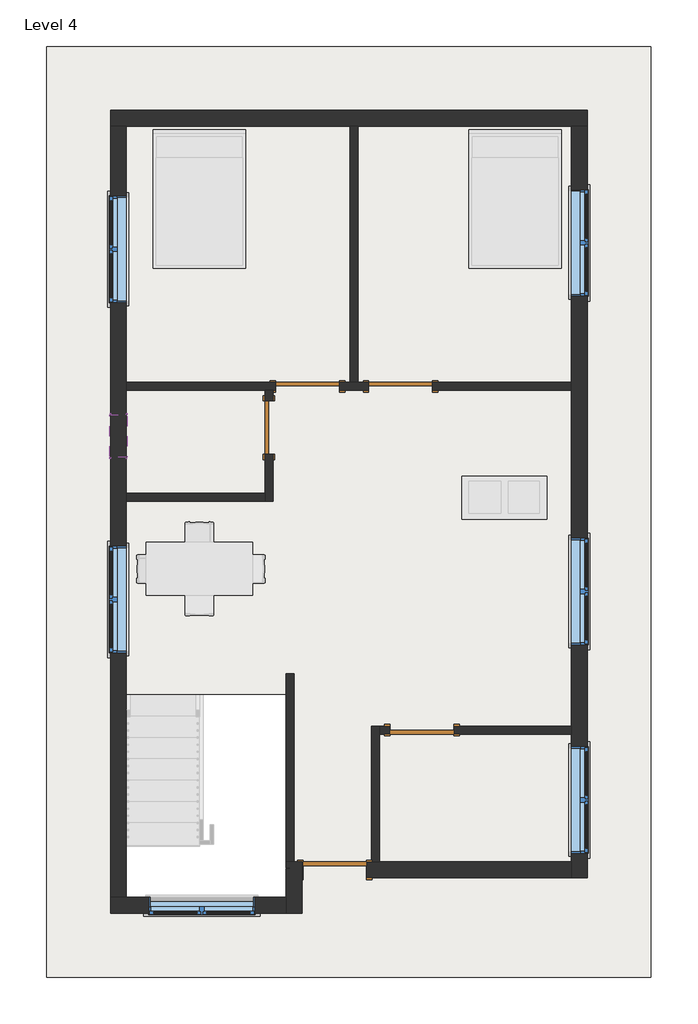
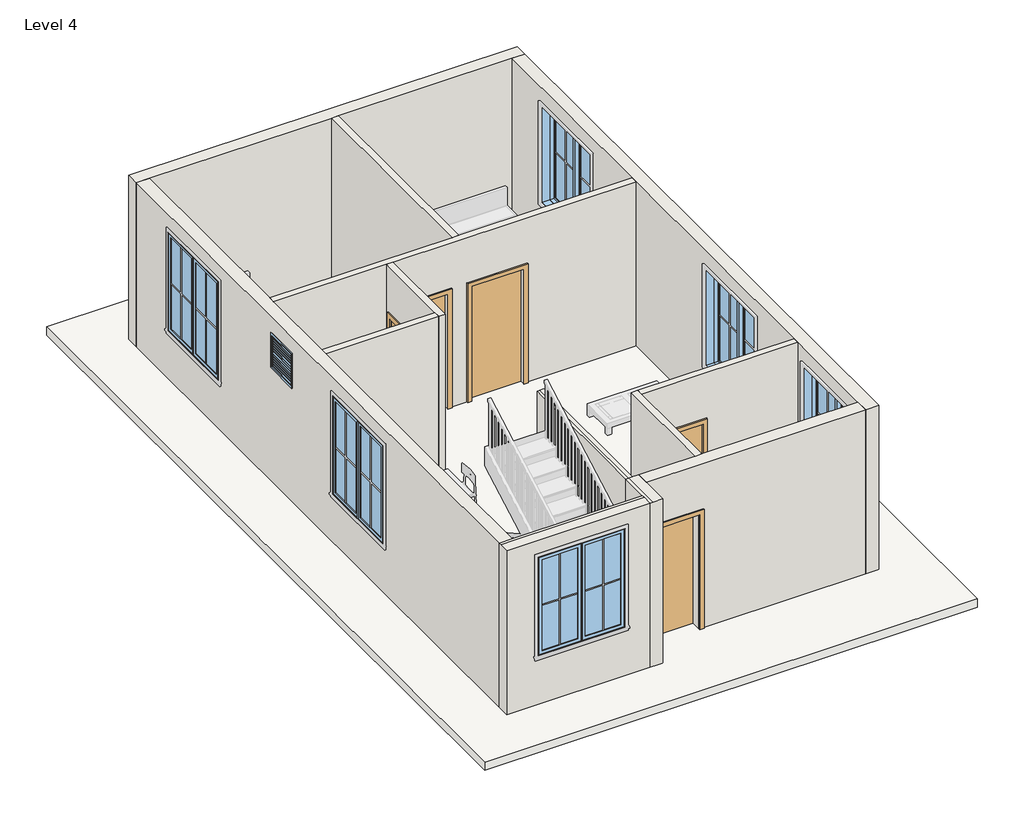
# One storey, part 1 of 3: 13 walls, 7 windows, 5 doors, 1 roof.
"""IFC4 building model written with IfcOpenShell, lengths in millimetres."""

from ifc_helpers import new_model, si_unit, frame, origin, place, context, project, spatial, polyline, outline, extrude, faceted_brep, transform, mapped, element, save
from components import door_214872d5, single_flush_door_3_e5f9f3c4, single_flush_door_3_305aa2a5, single_flush_door_3_0ca8825f, window_casement_double_win_5_f93960c7, window_f2d8fef0

model = new_model("IFC4")

# Units and contexts
model_context = context("Model", 3, world=origin())
ifc_project = project(units=[si_unit("LENGTHUNIT", "METRE", prefix="MILLI")], contexts=[model_context])

# Site, building, storey
site = spatial("IfcSite", under=ifc_project)
building = spatial("IfcBuilding", under=site)
storey = spatial("IfcBuildingStorey", under=building, Name="Level 4", Elevation=9448.8)

# Doors
placement = place(None, origin())
door_shape = door_214872d5(model_context)
element("IfcDoor", 1, ObjectType="Single-Flush : DOOR 2'6\"", at=placement, inside=storey, context=model_context, shape_type="MappedRepresentation", body=[
    mapped(door_shape, transform((-2193.930864, 251.0919982, 9448.8), x_axis=(0.0, 1.0, 0.0), y_axis=(-1.0, 0.0, 0.0), z_axis=(0.0, 0.0, 1.0))),
])
single_flush_door_3_shape = single_flush_door_3_e5f9f3c4(model_context)
element("IfcDoor", 2, ObjectType="Single-Flush : DOOR 3'", at=placement, inside=storey, context=model_context, shape_type="MappedRepresentation", body=[
    mapped(single_flush_door_3_shape, transform((-1641.3962678, 841.6419982, 9448.8), x_axis=(1.0, 0.0, 0.0), y_axis=(0.0, 1.0, 0.0), z_axis=(0.0, 0.0, 1.0))),
])
element("IfcDoor", 3, ObjectType="Single-Flush : DOOR 3'", at=placement, inside=storey, context=model_context, shape_type="MappedRepresentation", body=[
    mapped(single_flush_door_3_shape, transform((-3.180864, -4073.2580018, 9448.8), x_axis=(-1.0, 0.0, 0.0), y_axis=(0.0, -1.0, 0.0), z_axis=(0.0, 0.0, 1.0))),
])
single_flush_door_3_2_shape = single_flush_door_3_305aa2a5(model_context)
element("IfcDoor", 4, ObjectType="Single-Flush : DOOR 3'", at=placement, inside=storey, context=model_context, shape_type="MappedRepresentation", body=[
    mapped(single_flush_door_3_2_shape, transform((-307.980864, 841.6419982, 9448.8), x_axis=(-1.0, 0.0, 0.0), y_axis=(0.0, -1.0, 0.0), z_axis=(0.0, 0.0, 1.0))),
])
single_flush_door_3_3_shape = single_flush_door_3_0ca8825f(model_context)
element("IfcDoor", 5, ObjectType="Single-Flush : DOOR 3'", at=placement, inside=storey, context=model_context, shape_type="MappedRepresentation", body=[
    mapped(single_flush_door_3_3_shape, transform((-1250.955864, -6073.5080018, 9448.8), x_axis=(1.0, 0.0, 0.0), y_axis=(0.0, 1.0, 0.0), z_axis=(0.0, 0.0, 1.0))),
])

# Roof
element("IfcRoof", 6, ObjectType="ROOF 6\"", at=placement, inside=storey, context=model_context, shape_type="SweptSolid", body=[
    extrude(outline(polyline([(3273.419136, 5699.3919982), (3273.419136, -7610.2080018), (-5375.280864, -7610.2080018), (-5375.280864, 5699.3919982), (3273.419136, 5699.3919982)]), holes=[polyline([(-1895.480864, -3571.6080018), (-4232.280864, -3571.6080018), (-4232.280864, -6518.0080018), (-1895.480864, -6518.0080018), (-1895.480864, -3571.6080018)])]), frame((0.0, 0.0, 9296.4), z_axis=(0.0, 0.0, 1.0), x_axis=(1.0, 0.0, 0.0)), (0.0, 0.0, 1.0), 152.4),
])

# Walls
element("IfcWall", 7, ObjectType="WALL 4.5\"", at=placement, inside=storey, context=model_context, shape_type="SweptSolid", body=[
    extrude(outline(polyline([(-1031.880864, 898.7919982), (-1031.880864, 4556.3919982), (-917.580864, 4556.3919982), (-917.580864, 898.7919982), (-1031.880864, 898.7919982)])), frame((0.0, 0.0, 9448.8), z_axis=(0.0, 0.0, 1.0), x_axis=(1.0, 0.0, 0.0)), (0.0, 0.0, 1.0), 3048.0),
])
element("IfcWall", 8, ObjectType="WALL 4.5\"", at=placement, inside=storey, context=model_context, shape_type="Brep", body=[
    faceted_brep([(-765.180864, 898.7919982, 11582.4), (-765.180864, 898.7919982, 9448.8), (-917.580864, 898.7919982, 9448.8), (-1031.880864, 898.7919982, 9448.8), (-1184.1962678, 898.7919982, 9448.8), (-1184.1962678, 898.7919982, 11582.4), (-2098.5962678, 898.7919982, 11582.4), (-2098.5962678, 898.7919982, 9448.8), (-4232.280864, 898.7919982, 9448.8), (-4232.280864, 898.7919982, 12496.8), (-1031.880864, 898.7919982, 12496.8), (-917.580864, 898.7919982, 12496.8), (2130.419136, 898.7919982, 12496.8), (2130.419136, 898.7919982, 9448.8), (149.219136, 898.7919982, 9448.8), (149.219136, 898.7919982, 11582.4), (-1184.1962678, 784.4919982, 9448.8), (-765.180864, 784.4919982, 9448.8), (-765.180864, 784.4919982, 11582.4), (149.219136, 784.4919982, 11582.4), (149.219136, 784.4919982, 9448.8), (2130.419136, 784.4919982, 9448.8), (2130.419136, 784.4919982, 12496.8), (-2136.780864, 784.4919982, 12496.8), (-2251.080864, 784.4919982, 12496.8), (-4232.280864, 784.4919982, 12496.8), (-4232.280864, 784.4919982, 9448.8), (-2251.080864, 784.4919982, 9448.8), (-2136.780864, 784.4919982, 9448.8), (-2098.5962678, 784.4919982, 9448.8), (-2098.5962678, 784.4919982, 11582.4), (-1184.1962678, 784.4919982, 11582.4)], [[[0, 1, 2, 3, 4, 5, 6, 7, 8, 9, 10, 11, 12, 13, 14, 15]], [[16, 17, 18, 19, 20, 21, 22, 23, 24, 25, 26, 27, 28, 29, 30, 31]], [[29, 28, 27, 26, 8, 7]], [[14, 13, 21, 20]], [[4, 3, 2, 1, 17, 16]], [[13, 12, 22, 21]], [[9, 8, 26, 25]], [[5, 4, 16, 31]], [[6, 5, 31, 30]], [[7, 6, 30, 29]], [[18, 17, 1, 0]], [[19, 18, 0, 15]], [[20, 19, 15, 14]], [[12, 11, 10, 9, 25, 24, 23, 22]]]),
])
element("IfcWall", 9, ObjectType="WALL 4.5\"", at=placement, inside=storey, context=model_context, shape_type="Brep", body=[
    faceted_brep([(-2251.080864, 784.4919982, 9448.8), (-2251.080864, 632.0919982, 9448.8), (-2251.080864, 632.0919982, 11582.4), (-2251.080864, -129.9080018, 11582.4), (-2251.080864, -129.9080018, 9448.8), (-2251.080864, -688.7080018, 9448.8), (-2251.080864, -803.0080018, 9448.8), (-2251.080864, -803.0080018, 12496.8), (-2251.080864, -688.7080018, 12496.8), (-2251.080864, 784.4919982, 12496.8), (-2136.780864, 632.0919982, 11582.4), (-2136.780864, 632.0919982, 9448.8), (-2136.780864, 784.4919982, 9448.8), (-2136.780864, 784.4919982, 12496.8), (-2136.780864, -803.0080018, 12496.8), (-2136.780864, -803.0080018, 9448.8), (-2136.780864, -129.9080018, 9448.8), (-2136.780864, -129.9080018, 11582.4)], [[[0, 1, 2, 3, 4, 5, 6, 7, 8, 9]], [[10, 11, 12, 13, 14, 15, 16, 17]], [[16, 15, 6, 5, 4]], [[12, 11, 1, 0]], [[0, 9, 13, 12]], [[7, 6, 15, 14]], [[2, 1, 11, 10]], [[3, 2, 10, 17]], [[4, 3, 17, 16]], [[9, 8, 7, 14, 13]]]),
])
element("IfcWall", 10, ObjectType="WALL 4.5\"", at=placement, inside=storey, context=model_context, shape_type="SweptSolid", body=[
    extrude(outline(polyline([(-4232.280864, -688.7080018), (-2251.080864, -688.7080018), (-2251.080864, -803.0080018), (-4232.280864, -803.0080018), (-4232.280864, -688.7080018)])), frame((0.0, 0.0, 9448.8), z_axis=(0.0, 0.0, 1.0), x_axis=(1.0, 0.0, 0.0)), (0.0, 0.0, 1.0), 3048.0),
])
element("IfcWall", 11, ObjectType="WALL 4.5\"", at=placement, inside=storey, context=model_context, shape_type="Brep", body=[
    faceted_brep([(-1831.980864, -5959.2080018, 9448.8), (-1831.980864, -3266.8080018, 9448.8), (-1831.980864, -3266.8080018, 12496.8), (-1831.980864, -5959.2080018, 12496.8), (-1946.280864, -5959.2080018, 9448.8), (-1946.280864, -5959.2080018, 12496.8), (-1946.280864, -3266.8080018, 12496.8), (-1946.280864, -3266.8080018, 9448.8), (-1895.480864, -3266.8080018, 12496.8), (-1895.480864, -5959.2080018, 12496.8), (-1895.480864, -3571.6080018, 12496.8)], [[[0, 1, 2, 3]], [[4, 5, 6, 7]], [[1, 0, 4, 7]], [[2, 1, 7, 6, 8]], [[0, 3, 9, 5, 4]], [[3, 2, 8, 10, 9]], [[8, 6, 5, 9, 10]]]),
])
element("IfcWall", 12, ObjectType="WALL 4.5\"", at=placement, inside=storey, context=model_context, shape_type="Brep", body=[
    faceted_brep([(-612.780864, -5959.2080018, 9448.8), (-612.780864, -4130.4080018, 9448.8), (-612.780864, -4016.1080018, 9448.8), (-612.780864, -4016.1080018, 12496.8), (-612.780864, -4130.4080018, 12496.8), (-612.780864, -5959.2080018, 12496.8), (-727.080864, -5959.2080018, 9448.8), (-727.080864, -5959.2080018, 12496.8), (-727.080864, -4016.1080018, 12496.8), (-727.080864, -4016.1080018, 9448.8)], [[[0, 1, 2, 3, 4, 5]], [[6, 7, 8, 9]], [[2, 1, 0, 6, 9]], [[0, 5, 7, 6]], [[3, 2, 9, 8]], [[5, 4, 3, 8, 7]]]),
])
element("IfcWall", 13, ObjectType="WALL 4.5\"", at=placement, inside=storey, context=model_context, shape_type="SweptSolid", body=[
    extrude(outline(polyline([(9448.8, -612.780864), (9448.8, -460.380864), (11582.4, -460.380864), (11582.4, 454.019136), (9448.8, 454.019136), (9448.8, 2130.419136), (12496.8, 2130.419136), (12496.8, -612.780864), (9448.8, -612.780864)])), frame((0.0, -4130.4080018, 0.0), z_axis=(0.0, 1.0, 0.0), x_axis=(0.0, 0.0, 1.0)), (0.0, 0.0, 1.0), 114.3),
])
element("IfcWall", 14, ObjectType="WALL 9\"", at=placement, inside=storey, context=model_context, shape_type="Brep", body=[
    faceted_brep([(-4460.880864, 4556.3919982, 9448.8), (-4232.280864, 4556.3919982, 9448.8), (-1031.880864, 4556.3919982, 9448.8), (-917.580864, 4556.3919982, 9448.8), (2130.419136, 4556.3919982, 9448.8), (2359.019136, 4556.3919982, 9448.8), (2359.019136, 4556.3919982, 12496.8), (2130.419136, 4556.3919982, 12496.8), (-917.580864, 4556.3919982, 12496.8), (-1031.880864, 4556.3919982, 12496.8), (-4232.280864, 4556.3919982, 12496.8), (-4460.880864, 4556.3919982, 12496.8), (-4460.880864, 4784.9919982, 9448.8), (-4460.880864, 4784.9919982, 12496.8), (2359.019136, 4784.9919982, 12496.8), (2359.019136, 4784.9919982, 9448.8)], [[[0, 1, 2, 3, 4, 5, 6, 7, 8, 9, 10, 11]], [[12, 13, 14, 15]], [[5, 4, 3, 2, 1, 0, 12, 15]], [[6, 5, 15, 14]], [[0, 11, 13, 12]], [[11, 10, 9, 8, 7, 6, 14, 13]]]),
])
element("IfcWall", 15, ObjectType="WALL 9\"", at=placement, inside=storey, context=model_context, shape_type="Brep", body=[
    faceted_brep([(2130.419136, 4556.3919982, 9448.8), (2130.419136, 898.7919982, 9448.8), (2130.419136, 784.4919982, 9448.8), (2130.419136, -4016.1080018, 9448.8), (2130.419136, -4130.4080018, 9448.8), (2130.419136, -5959.2080018, 9448.8), (2130.419136, -6187.8080018, 9448.8), (2130.419136, -6187.8080018, 12496.8), (2130.419136, -5959.2080018, 12496.8), (2130.419136, -4130.4080018, 12496.8), (2130.419136, -4016.1080018, 12496.8), (2130.419136, 784.4919982, 12496.8), (2130.419136, 898.7919982, 12496.8), (2130.419136, 4556.3919982, 12496.8), (2130.419136, -5835.3830018, 12192.0), (2130.419136, -5835.3830018, 10363.2), (2130.419136, -4311.3830018, 10363.2), (2130.419136, -4311.3830018, 12192.0), (2130.419136, -2854.0580018, 12192.0), (2130.419136, -2854.0580018, 10363.2), (2130.419136, -1330.0580018, 10363.2), (2130.419136, -1330.0580018, 12192.0), (2130.419136, 2130.6919982, 12192.0), (2130.419136, 2130.6919982, 10363.2), (2130.419136, 3654.6919982, 10363.2), (2130.419136, 3654.6919982, 12192.0), (2359.019136, 4556.3919982, 9448.8), (2359.019136, 4556.3919982, 12496.8), (2359.019136, -6187.8080018, 12496.8), (2359.019136, -6187.8080018, 9448.8), (2359.019136, -5835.3830018, 12192.0), (2359.019136, -4311.3830018, 12192.0), (2359.019136, -4311.3830018, 10363.2), (2359.019136, -5835.3830018, 10363.2), (2359.019136, -2854.0580018, 12192.0), (2359.019136, -1330.0580018, 12192.0), (2359.019136, -1330.0580018, 10363.2), (2359.019136, -2854.0580018, 10363.2), (2359.019136, 2130.6919982, 12192.0), (2359.019136, 3654.6919982, 12192.0), (2359.019136, 3654.6919982, 10363.2), (2359.019136, 2130.6919982, 10363.2)], [[[0, 1, 2, 3, 4, 5, 6, 7, 8, 9, 10, 11, 12, 13], [14, 15, 16, 17], [18, 19, 20, 21], [22, 23, 24, 25]], [[26, 27, 28, 29], [30, 31, 32, 33], [34, 35, 36, 37], [38, 39, 40, 41]], [[6, 5, 4, 3, 2, 1, 0, 26, 29]], [[0, 13, 27, 26]], [[7, 6, 29, 28]], [[15, 14, 30, 33]], [[16, 15, 33, 32]], [[17, 16, 32, 31]], [[14, 17, 31, 30]], [[19, 18, 34, 37]], [[20, 19, 37, 36]], [[21, 20, 36, 35]], [[18, 21, 35, 34]], [[23, 22, 38, 41]], [[24, 23, 41, 40]], [[25, 24, 40, 39]], [[22, 25, 39, 38]], [[13, 12, 11, 10, 9, 8, 7, 28, 27]]]),
])
element("IfcWall", 16, ObjectType="WALL 9\"", at=placement, inside=storey, context=model_context, shape_type="Brep", body=[
    faceted_brep([(2130.419136, -5959.2080018, 9448.8), (-612.780864, -5959.2080018, 9448.8), (-727.080864, -5959.2080018, 9448.8), (-793.755864, -5959.2080018, 9448.8), (-793.755864, -5959.2080018, 11582.4), (-1708.155864, -5959.2080018, 11582.4), (-1708.155864, -5959.2080018, 9448.8), (-1717.680864, -5959.2080018, 9448.8), (-1717.680864, -5959.2080018, 12496.8), (-727.080864, -5959.2080018, 12496.8), (-612.780864, -5959.2080018, 12496.8), (2130.419136, -5959.2080018, 12496.8), (-793.755864, -6187.8080018, 11582.4), (-793.755864, -6187.8080018, 9448.8), (2130.419136, -6187.8080018, 9448.8), (2130.419136, -6187.8080018, 12496.8), (-1717.680864, -6187.8080018, 12496.8), (-1717.680864, -6187.8080018, 9448.8), (-1708.155864, -6187.8080018, 9448.8), (-1708.155864, -6187.8080018, 11582.4)], [[[0, 1, 2, 3, 4, 5, 6, 7, 8, 9, 10, 11]], [[12, 13, 14, 15, 16, 17, 18, 19]], [[18, 17, 7, 6]], [[14, 13, 3, 2, 1, 0]], [[0, 11, 15, 14]], [[8, 7, 17, 16]], [[4, 3, 13, 12]], [[5, 4, 12, 19]], [[6, 5, 19, 18]], [[11, 10, 9, 8, 16, 15]]]),
])
element("IfcWall", 17, ObjectType="WALL 9\"", at=placement, inside=storey, context=model_context, shape_type="Brep", body=[
    faceted_brep([(-1946.280864, -5959.2080018, 9448.8), (-1946.280864, -6467.2080018, 9448.8), (-1946.280864, -6695.8080018, 9448.8), (-1946.280864, -6695.8080018, 12496.8), (-1946.280864, -6467.2080018, 12496.8), (-1946.280864, -5959.2080018, 12496.8), (-1717.680864, -5959.2080018, 9448.8), (-1717.680864, -5959.2080018, 12496.8), (-1717.680864, -6187.8080018, 12496.8), (-1717.680864, -6695.8080018, 12496.8), (-1717.680864, -6695.8080018, 9448.8), (-1717.680864, -6187.8080018, 9448.8), (-1831.980864, -5959.2080018, 9448.8), (-1895.480864, -5959.2080018, 12496.8), (-1831.980864, -5959.2080018, 12496.8), (-1895.480864, -6695.8080018, 12496.8), (-1895.480864, -6518.0080018, 12496.8)], [[[0, 1, 2, 3, 4, 5]], [[6, 7, 8, 9, 10, 11]], [[2, 1, 0, 12, 6, 11, 10]], [[0, 5, 13, 14, 7, 6, 12]], [[3, 2, 10, 9, 15]], [[5, 4, 3, 15, 16, 13]], [[15, 9, 8, 7, 14, 13, 16]]]),
])
element("IfcWall", 18, ObjectType="WALL 9\"", at=placement, inside=storey, context=model_context, shape_type="Brep", body=[
    faceted_brep([(-1946.280864, -6467.2080018, 9448.8), (-4232.280864, -6467.2080018, 9448.8), (-4460.880864, -6467.2080018, 9448.8), (-4460.880864, -6467.2080018, 12496.8), (-4232.280864, -6467.2080018, 12496.8), (-1946.280864, -6467.2080018, 12496.8), (-3914.780864, -6467.2080018, 12192.0), (-3914.780864, -6467.2080018, 10363.2), (-2390.780864, -6467.2080018, 10363.2), (-2390.780864, -6467.2080018, 12192.0), (-1946.280864, -6695.8080018, 9448.8), (-1946.280864, -6695.8080018, 12496.8), (-4460.880864, -6695.8080018, 12496.8), (-4460.880864, -6695.8080018, 9448.8), (-3914.780864, -6695.8080018, 12192.0), (-2390.780864, -6695.8080018, 12192.0), (-2390.780864, -6695.8080018, 10363.2), (-3914.780864, -6695.8080018, 10363.2), (-1946.280864, -6518.0080018, 12496.8), (-4460.880864, -6518.0080018, 12496.8), (-4232.280864, -6518.0080018, 12496.8)], [[[0, 1, 2, 3, 4, 5], [6, 7, 8, 9]], [[10, 11, 12, 13], [14, 15, 16, 17]], [[2, 1, 0, 10, 13]], [[0, 5, 18, 11, 10]], [[3, 2, 13, 12, 19]], [[7, 6, 14, 17]], [[8, 7, 17, 16]], [[9, 8, 16, 15]], [[6, 9, 15, 14]], [[5, 4, 3, 19, 20, 18]], [[19, 12, 11, 18, 20]]]),
])
element("IfcWall", 19, ObjectType="WALL 9\"", at=placement, inside=storey, context=model_context, shape_type="Brep", body=[
    faceted_brep([(-4232.280864, -6467.2080018, 9448.8), (-4232.280864, -803.0080018, 9448.8), (-4232.280864, -688.7080018, 9448.8), (-4232.280864, 784.4919982, 9448.8), (-4232.280864, 898.7919982, 9448.8), (-4232.280864, 4556.3919982, 9448.8), (-4232.280864, 4556.3919982, 12496.8), (-4232.280864, 898.7919982, 12496.8), (-4232.280864, 784.4919982, 12496.8), (-4232.280864, -688.7080018, 12496.8), (-4232.280864, -803.0080018, 12496.8), (-4232.280864, -3571.6080018, 12496.8), (-4232.280864, -6467.2080018, 12496.8), (-4232.280864, -1445.1400081, 12192.0), (-4232.280864, -1445.1400081, 10363.2), (-4232.280864, -2969.1400081, 10363.2), (-4232.280864, -2969.1400081, 12192.0), (-4232.280864, 3562.6287133, 12192.0), (-4232.280864, 3562.6287133, 10363.2), (-4232.280864, 2038.6287133, 10363.2), (-4232.280864, 2038.6287133, 12192.0), (-4232.280864, -174.3580018, 12192.0), (-4232.280864, 435.2419982, 12192.0), (-4232.280864, 435.2419982, 11582.4), (-4232.280864, -174.3580018, 11582.4), (-4460.880864, -6467.2080018, 9448.8), (-4460.880864, -6467.2080018, 12496.8), (-4460.880864, 4556.3919982, 12496.8), (-4460.880864, 4556.3919982, 9448.8), (-4460.880864, -1445.1400081, 12192.0), (-4460.880864, -2969.1400081, 12192.0), (-4460.880864, -2969.1400081, 10363.2), (-4460.880864, -1445.1400081, 10363.2), (-4460.880864, 3562.6287133, 12192.0), (-4460.880864, 2038.6287133, 12192.0), (-4460.880864, 2038.6287133, 10363.2), (-4460.880864, 3562.6287133, 10363.2), (-4460.880864, -174.3580018, 12192.0), (-4460.880864, -174.3580018, 11582.4), (-4460.880864, 435.2419982, 11582.4), (-4460.880864, 435.2419982, 12192.0)], [[[0, 1, 2, 3, 4, 5, 6, 7, 8, 9, 10, 11, 12], [13, 14, 15, 16], [17, 18, 19, 20], [21, 22, 23, 24]], [[25, 26, 27, 28], [29, 30, 31, 32], [33, 34, 35, 36], [37, 38, 39, 40]], [[5, 4, 3, 2, 1, 0, 25, 28]], [[6, 5, 28, 27]], [[0, 12, 26, 25]], [[14, 13, 29, 32]], [[15, 14, 32, 31]], [[16, 15, 31, 30]], [[13, 16, 30, 29]], [[18, 17, 33, 36]], [[19, 18, 36, 35]], [[20, 19, 35, 34]], [[17, 20, 34, 33]], [[38, 37, 21, 24]], [[39, 38, 24, 23]], [[40, 39, 23, 22]], [[37, 40, 22, 21]], [[12, 11, 10, 9, 8, 7, 6, 27, 26]]]),
])

# Windows
window_casement_double_win_5_shape = window_casement_double_win_5_f93960c7(model_context)
element("IfcWindow", 20, ObjectType="Window-Casement-Double : WIN 5'", at=placement, inside=storey, context=model_context, shape_type="MappedRepresentation", body=[
    mapped(window_casement_double_win_5_shape, transform((-3152.780864, -6581.5080018, 9448.8), x_axis=(-1.0, 0.0, 0.0), y_axis=(0.0, -1.0, 0.0), z_axis=(0.0, 0.0, 1.0))),
])
element("IfcWindow", 21, ObjectType="Window-Casement-Double : WIN 5'", at=placement, inside=storey, context=model_context, shape_type="MappedRepresentation", body=[
    mapped(window_casement_double_win_5_shape, transform((2244.719136, -5073.3830018, 9448.8), x_axis=(0.0, -1.0, 0.0), y_axis=(1.0, 0.0, 0.0), z_axis=(0.0, 0.0, 1.0))),
])
element("IfcWindow", 22, ObjectType="Window-Casement-Double : WIN 5'", at=placement, inside=storey, context=model_context, shape_type="MappedRepresentation", body=[
    mapped(window_casement_double_win_5_shape, transform((2244.719136, -2092.0580018, 9448.8), x_axis=(0.0, -1.0, 0.0), y_axis=(1.0, 0.0, 0.0), z_axis=(0.0, 0.0, 1.0))),
])
element("IfcWindow", 23, ObjectType="Window-Casement-Double : WIN 5'", at=placement, inside=storey, context=model_context, shape_type="MappedRepresentation", body=[
    mapped(window_casement_double_win_5_shape, transform((-4346.580864, -2207.1400081, 9448.8), x_axis=(0.0, 1.0, 0.0), y_axis=(-1.0, 0.0, 0.0), z_axis=(0.0, 0.0, 1.0))),
])
element("IfcWindow", 24, ObjectType="Window-Casement-Double : WIN 5'", at=placement, inside=storey, context=model_context, shape_type="MappedRepresentation", body=[
    mapped(window_casement_double_win_5_shape, transform((2244.719136, 2892.6919982, 9448.8), x_axis=(0.0, -1.0, 0.0), y_axis=(1.0, 0.0, 0.0), z_axis=(0.0, 0.0, 1.0))),
])
element("IfcWindow", 25, ObjectType="Window-Casement-Double : WIN 5'", at=placement, inside=storey, context=model_context, shape_type="MappedRepresentation", body=[
    mapped(window_casement_double_win_5_shape, transform((-4346.580864, 2800.6287133, 9448.8), x_axis=(0.0, 1.0, 0.0), y_axis=(-1.0, 0.0, 0.0), z_axis=(0.0, 0.0, 1.0))),
])
window_shape = window_f2d8fef0(model_context)
element("IfcWindow", 26, ObjectType="Window-Louvers : 24\" x 24\"", at=placement, inside=storey, context=model_context, shape_type="MappedRepresentation", body=[
    mapped(window_shape, transform((-4352.930864, 130.4419982, 10668.0), x_axis=(0.0, 1.0, 0.0), y_axis=(-1.0, 0.0, 0.0), z_axis=(0.0, 0.0, 1.0))),
])

save(model, "model.ifc")

# Revit data of these elements
# Type "Single-Flush : DOOR 2'6\""
#   Type Mark = "9"
#   Construction Type Id = "MDOOR"
#   Assembly Code = "C1020"
#   Analytic Construction = "Metal"
#   Thickness = 0' - 2"
#   Heat Transfer Coefficient (U) = 0.651978 BTU/(h·ft²·°F)
#   Height = 7' - 0"
#   Trim Projection Ext = 0' - 1"
#   Trim Projection Int = 0' - 1"
#   Trim Width = 0' - 3"
#   Width = 2' - 6"
#   Define Thermal Properties by = 1
#   Door Material = Door - Panel
#   Frame Material = Door - Frame
#   Visual Light Transmittance = 0
#   Solar Heat Gain Coefficient = 0
#   Function = (empty or 0)
#   Wall Closure = (empty or 0)
# Type "Single-Flush : DOOR 3'"
#   Type Mark = "8"
#   Construction Type Id = "MDOOR"
#   Assembly Code = "C1020"
#   Analytic Construction = "Metal"
#   Thickness = 0' - 2"
#   Heat Transfer Coefficient (U) = 0.651978 BTU/(h·ft²·°F)
#   Height = 7' - 0"
#   Trim Projection Ext = 0' - 1"
#   Trim Projection Int = 0' - 1"
#   Trim Width = 0' - 3"
#   Width = 3' - 0"
#   Define Thermal Properties by = 1
#   Door Material = Door - Panel
#   Frame Material = Door - Frame
#   Visual Light Transmittance = 0
#   Solar Heat Gain Coefficient = 0
#   Function = (empty or 0)
#   Wall Closure = (empty or 0)
# Type "ROOF 6\""
#   Assembly Code = "B1020"
#   Layers, outside or top first: 0' - 6" no material (function 1)
# Type "WALL 4.5\""
#   Assembly Code = "B2010"
#   Layers, outside or top first: 0' - 4 1/2" no material (function 1)
# Type "WALL 9\""
#   Assembly Code = "B2010"
#   Layers, outside or top first: 0' - 9" no material (function 1)
# Type "Window-Casement-Double : WIN 5'"
#   Type Mark = "18"
#   Fire Rating = "0.5h"
#   Assembly Code = "B2020100"
#   Analytic Construction = "Double glazing - domestic"
#   Frame Extension [instance default] = 0' - 0 1/4"
#   Window Inset [instance default] = 0' - 0"
#   Wall Thickness [instance default] = 0' - 6"
#   Interior Wall Closure [instance default] = 0' - 2 1/4"
#   Half Width = 2' - 6"
#   Visual Light Transmittance = 0.81
#   Thermal Resistance (R) = 1.8146 (h·ft²·°F)/BTU
#   Solar Heat Gain Coefficient = 0.76
#   Rough Width = 5' - 0 1/2"
#   Rough Height = 6' - 0 1/2"
#   Height = 6' - 0"
#   Heat Transfer Coefficient (U) = 0.5511 BTU/(h·ft²·°F)
#   Exterior Wall Closure [instance default] = 0' - 1 1/4"
#   Extension Jamb [instance default] = 0' - 2 1/4"
#   Default Sill Height = 3' - 0"
#   Width = 5' - 0"
#   Muntin Visibility = yes
#   Interior Trim Visibility [instance default] = yes
#   Exterior Trim Visibility [instance default] = yes
#   Extension Jamb Visibility [instance default] = yes
#   Interior Trim Material = Wood - Stained
#   Muntin Pattern = Muntin Pattern_2x2 : Muntin Pattern_2x2
#   Interior Trim = Trim-Window-Interior-Flat : Picture Frame
#   Interior Frame Material = Wood - Stained
#   Glass Panel Material = Glass
#   Exterior Trim Material = Clad - White
#   Exterior Trim = Trim-Window-Exterior-Flat : with Sill
#   Exterior Frame Material = Clad - White
#   Wall Closure = (empty or 0)
# Type "Window-Louvers : 24\" x 24\""
#   Type Mark = "19"
#   Construction Type Id = "GSP4R"
#   Assembly Code = "B20"
#   Analytic Construction = "1/8 in Pilkington single glazing"
#   Visual Light Transmittance = 0.9
#   Thermal Resistance (R) = 1.53941 (h·ft²·°F)/BTU
#   Solar Heat Gain Coefficient = 0.78
#   Max Height = 1' - 11.74264"
#   Height = 2' - 0"
#   Heat Transfer Coefficient (U) = 0.6496 BTU/(h·ft²·°F)
#   Blade Width [instance default] = 1' - 10 1/2"
#   Blade Vertical Thickness = 0' - 0.35355"
#   Blade Thickness = 0' - 0 1/4"
#   Blade Spacing = 0' - 1 1/2"
#   Blade Height = 0' - 1.85355"
#   Blade Depth = 0' - 3"
#   Blade Angle = 45.00°
#   Default Sill Height = 3' - 0"
#   Trim Projection_Exterior = 0' - 0 1/2"
#   Trim Projection_Interior = 0' - 0 1/2"
#   Trim Width_Exterior = 0' - 1 1/2"
#   Trim Width_Interior = 0' - 1 1/2"
#   Width = 2' - 0"
#   Max Blade Count = 12
#   Define Thermal Properties by = 1
#   Blade Count = 12
#   Frame Material = Birch
#   Louver Material = Birch
#   Trim Exterior Material = Birch
#   Trim Interior Material = Birch
#   Wall Closure = (empty or 0)
# Element 1 (IfcDoor, "Single-Flush : DOOR 2'6\"")
#   Phase Created = New Construction
#   Materials on its faces: "Door - Frame", "Door - Panel"
# Elements 2, 3, 4, 5 (IfcDoor, "Single-Flush : DOOR 3'")
#   Phase Created = New Construction
#   Materials on its faces: "Door - Frame", "Door - Panel"
# Element 6 (IfcRoof, "ROOF 6\"")
#   built-in parameter 1001705 = 31 (stored number, unit not read)
#   built-in parameter 1001701 = -0.5 (stored number, unit not read)
#   built-in parameter 1001710 = 33615
#   Phase Created = New Construction
#   Materials on its faces: "Copper", "Wood - Stained"
# Elements 7, 8, 9, 10, 12, 13 (IfcWall, "WALL 4.5\"")
#   Top Offset = 0' - 0"
#   Base Offset = 0' - 0"
#   Unconnected Height = 10' - 0"
#   wall height = 10' - 0"
#   Phase Created = New Construction
#   Base Constraint = Level 4
#   Materials on its faces: "Default Wall"
# Element 11 (IfcWall, "WALL 4.5\"")
#   Top Offset = 0' - 0"
#   Base Offset = 0' - 0"
#   Unconnected Height = 10' - 0"
#   wall height = 10' - 0"
#   Phase Created = New Construction
#   Base Constraint = Level 4
#   Materials on its faces: "Default Wall", "Copper"
# Elements 14, 15, 16 (IfcWall, "WALL 9\"")
#   Top Offset = 0' - 0"
#   Base Offset = 0' - 0"
#   Unconnected Height = 10' - 0"
#   wall height = 10' - 0"
#   Phase Created = New Construction
#   Base Constraint = Level 4
#   Materials on its faces: "Default Wall"
# Elements 17, 18, 19 (IfcWall, "WALL 9\"")
#   Top Offset = 0' - 0"
#   Base Offset = 0' - 0"
#   Unconnected Height = 10' - 0"
#   wall height = 10' - 0"
#   Phase Created = New Construction
#   Base Constraint = Level 4
#   Materials on its faces: "Default Wall", "Copper"
# Element 20 (IfcWindow, "Window-Casement-Double : WIN 5'")
#   Mark = "22"
#   Window Inset = 0' - 0"
#   Interior Wall Closure = 0' - 2 1/4"
#   Frame Extension = 0' - 0 1/4"
#   Exterior Wall Closure = 0' - 1 1/4"
#   Interior Trim Visibility = yes
#   Exterior Trim Visibility = yes
#   Phase Created = New Construction
#   Materials on its faces: "Wood - Stained", "Glass", "Clad - White"
# Element 21 (IfcWindow, "Window-Casement-Double : WIN 5'")
#   Mark = "23"
#   Window Inset = 0' - 0"
#   Interior Wall Closure = 0' - 2 1/4"
#   Frame Extension = 0' - 0 1/4"
#   Exterior Wall Closure = 0' - 1 1/4"
#   Interior Trim Visibility = yes
#   Exterior Trim Visibility = yes
#   Phase Created = New Construction
#   Materials on its faces: "Wood - Stained", "Glass", "Clad - White"
# Element 22 (IfcWindow, "Window-Casement-Double : WIN 5'")
#   Mark = "24"
#   Window Inset = 0' - 0"
#   Interior Wall Closure = 0' - 2 1/4"
#   Frame Extension = 0' - 0 1/4"
#   Exterior Wall Closure = 0' - 1 1/4"
#   Interior Trim Visibility = yes
#   Exterior Trim Visibility = yes
#   Phase Created = New Construction
#   Materials on its faces: "Wood - Stained", "Glass", "Clad - White"
# Element 23 (IfcWindow, "Window-Casement-Double : WIN 5'")
#   Mark = "25"
#   Window Inset = 0' - 0"
#   Interior Wall Closure = 0' - 2 1/4"
#   Frame Extension = 0' - 0 1/4"
#   Exterior Wall Closure = 0' - 1 1/4"
#   Interior Trim Visibility = yes
#   Exterior Trim Visibility = yes
#   Phase Created = New Construction
#   Materials on its faces: "Wood - Stained", "Glass", "Clad - White"
# Element 24 (IfcWindow, "Window-Casement-Double : WIN 5'")
#   Mark = "26"
#   Window Inset = 0' - 0"
#   Interior Wall Closure = 0' - 2 1/4"
#   Frame Extension = 0' - 0 1/4"
#   Exterior Wall Closure = 0' - 1 1/4"
#   Interior Trim Visibility = yes
#   Exterior Trim Visibility = yes
#   Phase Created = New Construction
#   Materials on its faces: "Wood - Stained", "Glass", "Clad - White"
# Element 25 (IfcWindow, "Window-Casement-Double : WIN 5'")
#   Mark = "27"
#   Window Inset = 0' - 0"
#   Interior Wall Closure = 0' - 2 1/4"
#   Frame Extension = 0' - 0 1/4"
#   Exterior Wall Closure = 0' - 1 1/4"
#   Interior Trim Visibility = yes
#   Exterior Trim Visibility = yes
#   Phase Created = New Construction
#   Materials on its faces: "Wood - Stained", "Glass", "Clad - White"
# Element 26 (IfcWindow, "Window-Louvers : 24\" x 24\"")
#   Mark = "28"
#   Blade Width = 1' - 10 1/2"
#   Phase Created = New Construction
#   Materials on its faces: "Birch"
# Materials
#   "Door - Panel": class "Wood", colour RGB 210 159 95, transparency 0, Cost = 0
#   "Door - Frame": colour RGB 118 70 51, transparency 0, Cost = 0
#   "Wood - Stained": class "Wood", colour RGB 224 178 126, transparency 0, Cost = 0
#   "Glass": class "Glass", colour RGB 0 128 192, transparency 0.75, Description = "Soda Lime Glass", Cost = 0
#   "Clad - White": class "Wood", colour RGB 242 242 238, transparency 0, Cost = 0
#   "Birch": class "Wood", colour RGB 224 178 126, transparency 0, Description = "Betula Alleghaniensis", Cost = 0
#   "Copper": class "Metal", colour RGB 0 0 0, transparency 0, Description = "Copper, matte finish", Cost = 0
#   "Default Wall": colour RGB 128 128 128, transparency 0, Cost = 0
